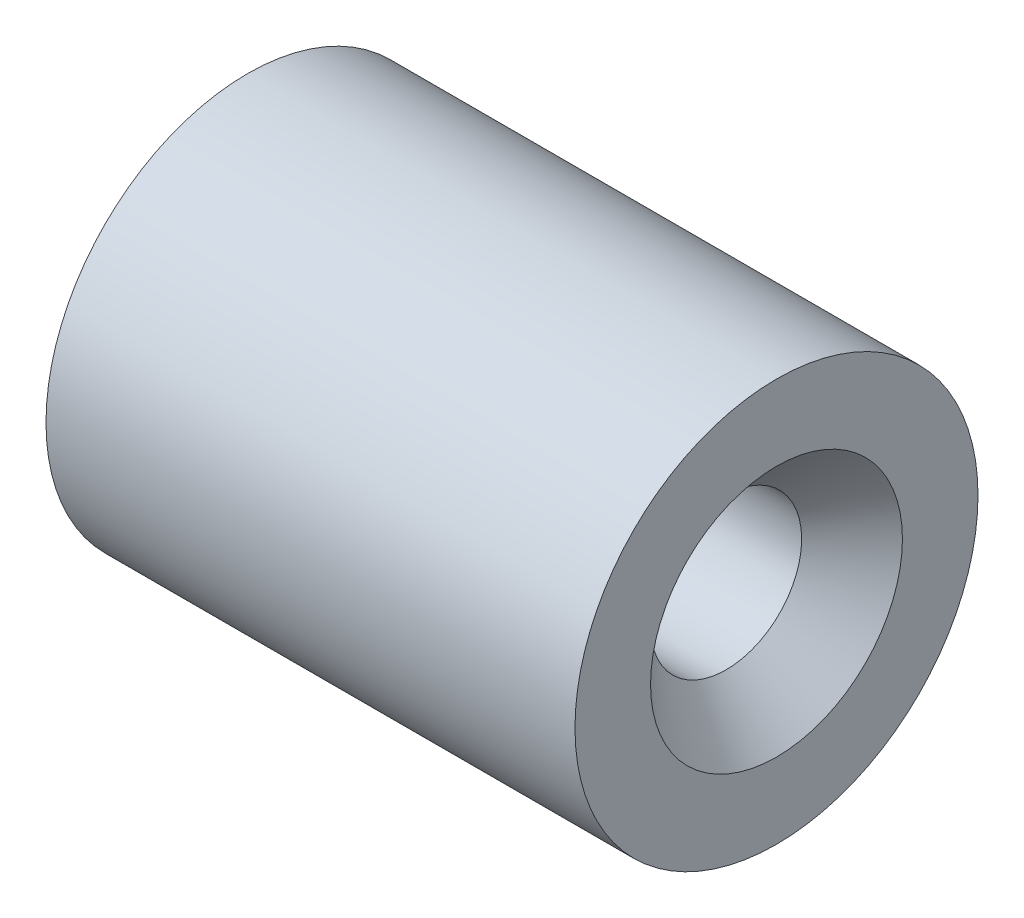
SolidWorks part; units mm, degrees
material "Plain Carbon Steel"
ref_plane "Front Plane" through (0, 0, 0) normal (0, 0, 1) x (1, 0, 0)
ref_plane "Top Plane" through (0, 0, 0) normal (0, 1, 0) x (1, 0, 0)
ref_plane "Right Plane" through (0, 0, 0) normal (1, 0, 0) x (0, 0, -1)
sketch "Bush Profile Sketch" plane through (0, 0, 0) normal (0, 0, 1) x (1, 0, 0)
  line L0 (0, 0) -> (-42, 0) construction
  line L1 (0, 10) -> (-4, 6)
  line L2 (-4, 6) -> (-38, 6)
  line L3 (-38, 6) -> (-42, 10)
  line L4 (-42, 10) -> (-42, 16)
  line L5 (-42, 16) -> (0, 16)
  line L6 (0, 16) -> (0, 10)
  line L7 (-4, 6) -> (9.2472, 6) construction
  line L8 (-38, 6) -> (-45.2948, 6) construction
  dimension "D1" = 42
  dimension "D2" = 45
  dimension "D3" = 16
  dimension "D4" = 6
  dimension "D5" = 10
  dimension "D6" = 45
revolve "Bush Body" add sketch "Bush Profile Sketch" angle 360 about L0
sketch "Internal Cut Profile Sketch" plane through (0, 0, 0) normal (0, 0, 1) x (1, 0, 0)
  line L0 (-21, 0) -> (-21, -23.2164) construction
  line L1 (-26.1962, -16) -> (-21, -13)
  line L2 (-42, -16) -> (0, -16) construction
  line L3 (-26.1962, -16) -> (-21, -16)
  line L4 (-21, -16) -> (-21, -13)
  dimension "D1" = 21
  dimension "D2" = 3
  dimension "D3" = 60
revolve "Internal Revolved Cut" cut sketch "Internal Cut Profile Sketch" angle 360 about L0
